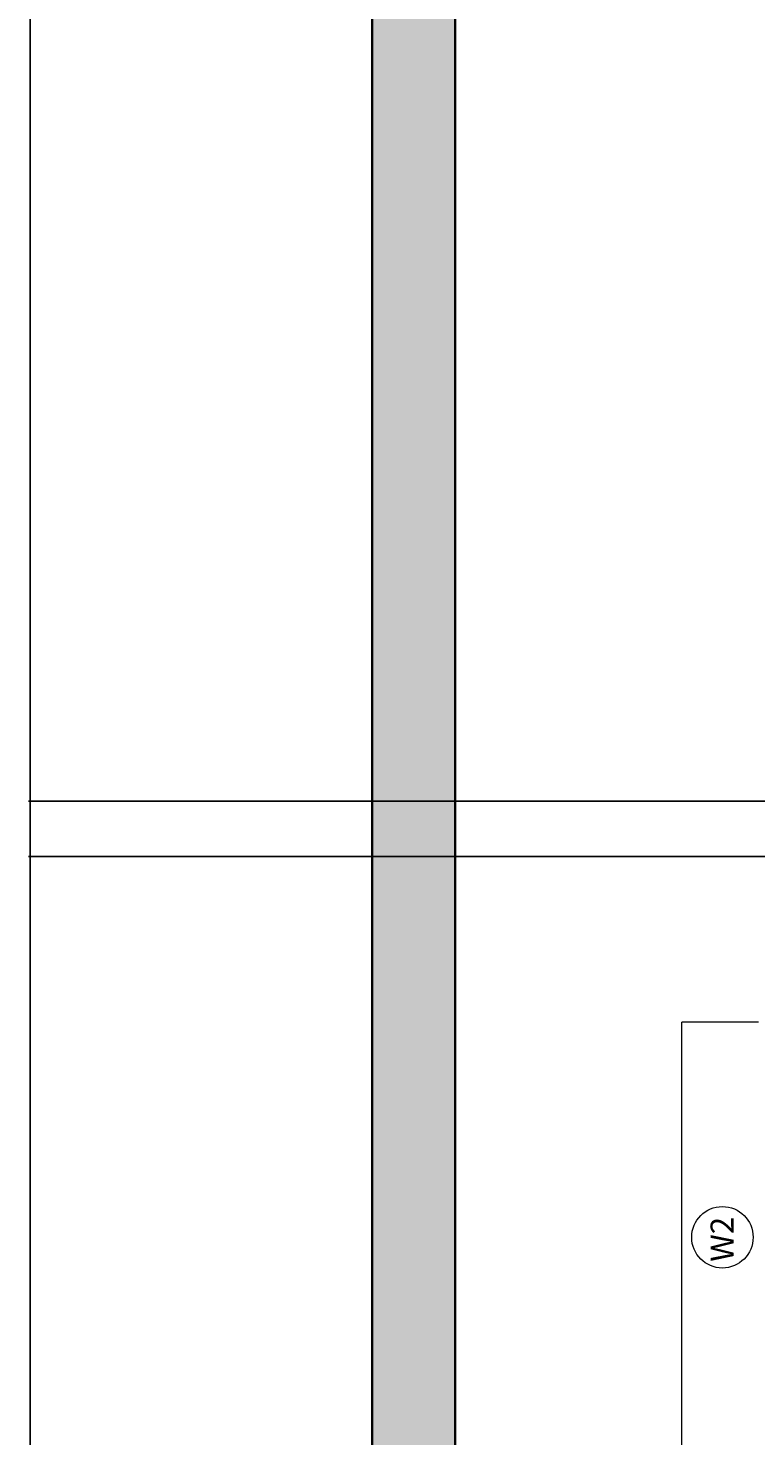
# Model space of a CAD drawing. Units: inches. Extents: x 2701 to 6846, y 811 to 2447.
# Tile 8 of 20: x 2701 to 2780, y 1309 to 1462. Entities that reach past the tile are written whole.
import ezdxf

# ---------------------------------------------------------------- set-up
doc = ezdxf.new("R2010")
doc.units = ezdxf.units.IN
for name, color, linetype, lineweight in [('A-ANNO-DIMS', 2, 'Continuous', 18), ('A-ANNO-IDEN', 7, 'Continuous', 13), ('A-GLAZ', 4, 'Continuous', 18), ('C-PROP', 7, 'Continuous', 35)]:
    doc.layers.add(name, color=color, linetype=linetype, lineweight=lineweight)
doc.layers.add('C-PROP-PATT', color=18, linetype='Continuous', lineweight=13, true_color=0x000000)
doc.styles.get("Standard").update_dxf_attribs({"font": 'arial.ttf'})
doc.dimstyles.get("Standard").update_dxf_attribs({"dimtxt": 0.18, "dimasz": 0.18, "dimexe": 0.18, "dimexo": 0.0625, "dimgap": 0.09, "dimtad": 0, "dimtih": 1, "dimtoh": 1, "dimdec": 4, "dimzin": 0, "dimdsep": 46, "dimtxsty": 'Standard', "dimcen": 0.09, "dimadec": 0, "dimazin": 0, "dimtfac": 1, "dimtdec": 4, "dimtofl": 0, "dimtmove": 0, "dimatfit": 3, "dimfxl": 1, "dimtolj": 1, "dimtzin": 0, "dimarcsym": 0})

# ---------------------------------------------------------------- blocks, each defined once
blk = doc.blocks.new('*D66')
at = {"layer": 'A-ANNO-DIMS', "color": 0, "lineweight": -2, "transparency": 16777216}
for p, q in [((2737.91, 1504.05), (2700.59, 1504.05)), ((2700.77, 1503.87), (2700.77, 1180.23)), ((2700.77, 856.23), (2700.77, 1179.87)), ((2737.91, 856.05), (2700.59, 856.05))]:
    blk.add_line(p, q, dxfattribs=at)
at = {"layer": 'A-ANNO-DIMS', "color": 0, "transparency": 16777216}
for points in [[(2700.74, 1503.87), (2700.8, 1503.87), (2700.77, 1504.05)], [(2700.74, 856.23), (2700.8, 856.23), (2700.77, 856.05)]]:
    blk.add_solid(points, dxfattribs=at)
at = {"layer": 'Defpoints', "color": 0, "transparency": 16777216}
for p in [(2700.77, 1504.05), (2737.97, 1504.05), (2737.97, 856.05)]:
    blk.add_point(p, dxfattribs=at)
at = {"layer": 'A-ANNO-DIMS', "color": 0, "transparency": 16777216, "insert": (2700.77, 1180.05), "char_height": 0.18, "attachment_point": 5}
blk.add_mtext('\\A1;648', dxfattribs=at)
blk = doc.blocks.new('*D75')
at = {"layer": 'A-ANNO-DIMS', "color": 0, "lineweight": -2, "transparency": 16777216}
for p, q in [((2923.91, 1378.05), (2700.59, 1378.05)), ((2700.77, 1377.87), (2700.77, 1375.23)), ((2700.77, 1372.23), (2700.77, 1374.87)), ((2923.91, 1372.05), (2700.59, 1372.05))]:
    blk.add_line(p, q, dxfattribs=at)
at = {"layer": 'A-ANNO-DIMS', "color": 0, "transparency": 16777216}
for points in [[(2700.74, 1377.87), (2700.8, 1377.87), (2700.77, 1378.05)], [(2700.74, 1372.23), (2700.8, 1372.23), (2700.77, 1372.05)]]:
    blk.add_solid(points, dxfattribs=at)
at = {"layer": 'Defpoints', "color": 0, "transparency": 16777216}
for p in [(2700.77, 1378.05), (2923.97, 1378.05), (2923.97, 1372.05)]:
    blk.add_point(p, dxfattribs=at)
at = {"layer": 'A-ANNO-DIMS', "color": 0, "transparency": 16777216, "insert": (2700.77, 1375.05), "char_height": 0.18, "attachment_point": 5}
blk.add_mtext('\\A1;6', dxfattribs=at)

msp = doc.modelspace()

# ---------------------------------------------------------------- hatches: boundary and pattern name
at = {"layer": 'C-PROP-PATT'}
h = msp.add_hatch(color=256, dxfattribs=at)
h.dxf.hatch_style = 1
h.paths.add_polyline_path([(3145.97, 1504.05), (2737.97, 1504.05), (2737.97, 967.05), (2746.97, 967.05), (2746.97, 1495.05), (3136.97, 1495.05), (3136.97, 865.05), (3130.97, 865.05), (3130.97, 856.05), (3145.97, 856.05)])
h.paths.add_polyline_path([(3070.97, 865.05), (2746.97, 865.05), (2746.97, 871.05), (2737.97, 871.05), (2737.97, 856.05), (3070.97, 856.05)], flags=17)

# ---------------------------------------------------------------- linework, layer by layer
at = {"layer": 'A-ANNO-IDEN'}
msp.add_circle((2776.04, 1330.66), 3.34, dxfattribs=at)
at = {"layer": 'A-GLAZ'}
for p in [(2771.64, 1306.05), (2779.97, 1354.05)]:
    msp.add_line(p, (2771.64, 1354.05), dxfattribs=at)
at = {"layer": 'C-PROP'}
for p, q in [((2737.97, 919.05), (2737.97, 1504.05)), ((2746.97, 967.05), (2746.97, 1495.05))]:
    msp.add_line(p, q, dxfattribs=at)

# ---------------------------------------------------------------- texts
at = {"layer": 'A-ANNO-IDEN', "insert": (2774.75, 1328), "char_height": 2.5, "attachment_point": 1, "rotation": 90}
msp.add_mtext_dynamic_manual_height_columns('W2', width=0.4422, gutter_width=12.5, heights=[0], dxfattribs=at)

# ---------------------------------------------------------------- dimensions: what is measured, and where the dimension line sits
at = {"layer": 'A-ANNO-DIMS'}
for base, p1, p2, picture, middle in [((2700.77, 1504.05), (2737.97, 856.05), (2737.97, 1504.05), '*D66', (2700.77, 1180.05)), ((2700.77, 1378.05), (2923.97, 1372.05), (2923.97, 1378.05), '*D75', (2700.77, 1375.05))]:
    dim = msp.add_linear_dim(base=base, p1=p1, p2=p2, angle=90, dimstyle='Standard', override={"dimdec": 0, "dimlfac": 1, "dimrnd": 0, "dimzin": 0, "dimdsep": 46, "dimlunit": 2}, dxfattribs=at)
    dim.commit()
    dim.dimension.update_dxf_attribs({"geometry": picture, "text_midpoint": middle})

doc.saveas('drawing.dxf')
